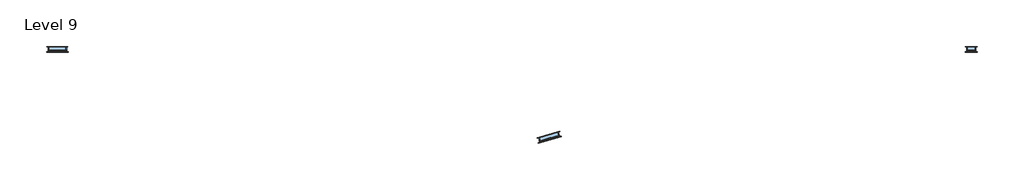
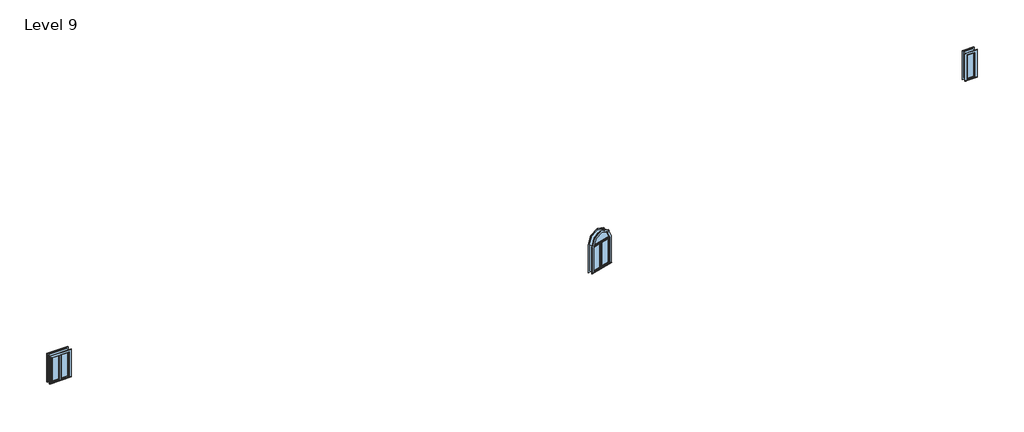
# One storey: 3 windows.
"""IFC4 building model written with IfcOpenShell, lengths in millimetres."""

from ifc_helpers import new_model, si_unit, origin, place, context, project, spatial, transform, mapped, element, save
from components import window_cf4adaea, window_a765b88f, window_bb17773d

model = new_model("IFC4")

# Units and contexts
model_context = context("Model", 3, world=origin())
ifc_project = project(units=[si_unit("LENGTHUNIT", "METRE", prefix="MILLI")], contexts=[model_context])

# Site, building, storey
site = spatial("IfcSite", under=ifc_project)
building = spatial("IfcBuilding", under=site)
storey = spatial("IfcBuildingStorey", under=building, Name="Level 9", Elevation=16154.4)

# Windows
placement = place(None, origin())
window_shape = window_cf4adaea(model_context)
element("IfcWindow", 1, ObjectType="36\" x 48\"", at=placement, inside=storey, context=model_context, shape_type="MappedRepresentation", body=[
    mapped(window_shape, transform((2850.7182758, -16224.4052953, 16154.4), x_axis=(-0.9600407790714355, -0.2798601481453037, 0.0), y_axis=(0.2798601481453037, -0.9600407790714355, 0.0), z_axis=(0.0, 0.0, 1.0))),
])
window_2_shape = window_a765b88f(model_context)
element("IfcWindow", 2, ObjectType="Awning with Trim : 16\" x 48\"", at=placement, inside=storey, context=model_context, shape_type="MappedRepresentation", body=[
    mapped(window_2_shape, transform((21425.814721, -12354.7237084, 16154.4), x_axis=(-1.0, 0.0, 0.0), y_axis=(0.0, -1.0, 0.0), z_axis=(0.0, 0.0, 1.0))),
])
window_3_shape = window_bb17773d(model_context)
element("IfcWindow", 3, ObjectType="Casement Dbl with Trim : 32\" x 48\"", at=placement, inside=storey, context=model_context, shape_type="MappedRepresentation", body=[
    mapped(window_3_shape, transform((-18807.785279, -12335.6737084, 16154.4), x_axis=(-1.0, 0.0, 0.0), y_axis=(0.0, -1.0, 0.0), z_axis=(0.0, 0.0, 1.0))),
])

save(model, "model.ifc")

# Revit data of these elements
# Type "36\" x 48\""
#   Type Mark = "38"
#   Construction Type Id = "SGL"
#   Assembly Code = "B2020100"
#   Analytic Construction = "Large single-glazed windows"
#   Visual Light Transmittance = 0.9
#   Solar Heat Gain Coefficient = 0.86
#   Heat Transfer Coefficient (U) = 0.979472 BTU/(h·ft²·°F)
#   Height = 4' - 0"
#   Default Sill Height = 3' - 0"
#   Trim Projection - Ext. = 0' - 0 1/2"
#   Trim Projection - Int. = 0' - 0 3/4"
#   Trim Width - Exterior = 0' - 3 1/2"
#   Trim Width - Interior = 0' - 3 1/2"
#   Width = 3' - 0"
#   Window Inset = 0' - 0 3/4"
#   Define Thermal Properties by = 1
#   Glass Pane Material = Glass
#   Sash Material = Sash
#   Trim Exterior Material = Trim
#   Trim Interior Material = Trim
#   Wall Closure = (empty or 0)
# Type "Awning with Trim : 16\" x 48\""
#   Type Mark = "14"
#   Construction Type Id = "GSP4R"
#   Assembly Code = "B2020100"
#   Analytic Construction = "1/8 in Pilkington single glazing"
#   Visual Light Transmittance = 0.9
#   Solar Heat Gain Coefficient = 0.78
#   Heat Transfer Coefficient (U) = 0.6496 BTU/(h·ft²·°F)
#   Height = 4' - 0"
#   Default Sill Height = 3' - 0"
#   Trim Projection - Ext. = 0' - 0 1/2"
#   Trim Projection - Int. = 0' - 0 3/4"
#   Trim Width - Exterior = 0' - 3 1/2"
#   Trim Width - Interior = 0' - 3 1/2"
#   Width = 1' - 4"
#   Window Inset = 0' - 0 3/4"
#   Define Thermal Properties by = 1
#   Glass Pane Material = Glass
#   Sash Material = Sash
#   Trim Exterior Material = Trim
#   Trim Interior Material = Trim
#   Wall Closure = (empty or 0)
# Type "Casement Dbl with Trim : 32\" x 48\""
#   Type Mark = "36"
#   Construction Type Id = "GSP4R"
#   Assembly Code = "B2020100"
#   Analytic Construction = "1/8 in Pilkington single glazing"
#   Visual Light Transmittance = 0.9
#   Solar Heat Gain Coefficient = 0.78
#   Heat Transfer Coefficient (U) = 0.6496 BTU/(h·ft²·°F)
#   Height = 4' - 0"
#   Default Sill Height = 3' - 0"
#   Trim Projection - Ext. = 0' - 0 1/2"
#   Trim Projection - Int. = 0' - 0 3/4"
#   Trim Width - Exterior = 0' - 3 1/2"
#   Trim Width - Interior = 0' - 3 1/2"
#   Width = 2' - 8"
#   Window Inset = 0' - 0 3/4"
#   Define Thermal Properties by = 1
#   Glass Pane Material = Glass
#   Sash Material = Sash
#   Trim Exterior Material = Trim
#   Trim Interior Material = Trim
#   Wall Closure = (empty or 0)
# Element 1 (IfcWindow, "36\" x 48\"")
#   Mark = "29"
#   Phase Created = New Construction
#   Materials on its faces: "Sash", "Trim", "Glass"
# Element 2 (IfcWindow, "Awning with Trim : 16\" x 48\"")
#   Mark = "63"
#   Phase Created = New Construction
#   Materials on its faces: "Sash", "Trim", "Glass"
# Element 3 (IfcWindow, "Casement Dbl with Trim : 32\" x 48\"")
#   Mark = "46"
#   Phase Created = New Construction
#   Materials on its faces: "Sash", "Trim", "Glass"
# Materials
#   "Glass": class "Glass", colour RGB 0 128 192, transparency 0.75, Description = "Soda Lime Glass", Cost = 0
#   "Sash": class "Wood", colour RGB 224 178 126, transparency 0
#   "Trim": class "Wood", colour RGB 224 178 126, transparency 0
